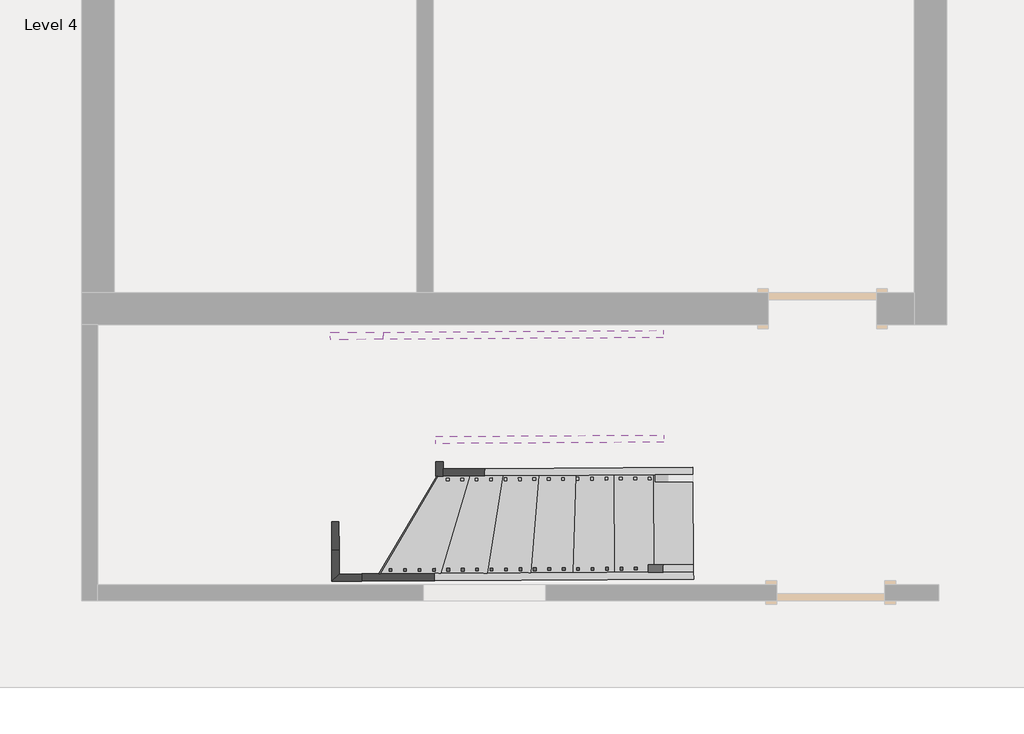
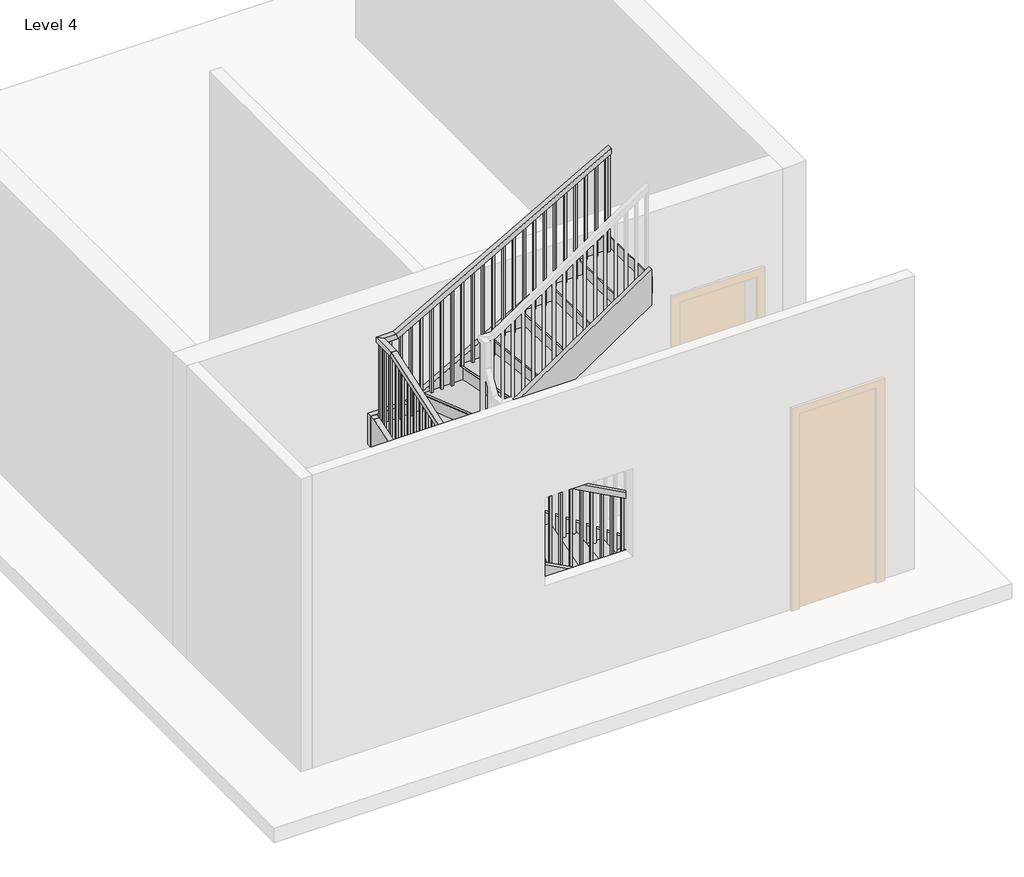
# One storey, part 2 of 2: 9 members, 1 railing, 1 stair flight.
"""IFC4 building model written with IfcOpenShell, lengths in millimetres."""

from ifc_helpers import new_model, si_unit, frame, origin, place, context, project, spatial, polyline, outline, extrude, faceted_brep, transform, mapped, element, save
from components import stair_flight_a1ba2c50

model = new_model("IFC4")

# Units and contexts
model_context = context("Model", 3, world=origin())
ifc_project = project(units=[si_unit("LENGTHUNIT", "METRE", prefix="MILLI")], contexts=[model_context])

# Site, building, storey
site = spatial("IfcSite", under=ifc_project)
building = spatial("IfcBuilding", under=site)
storey = spatial("IfcBuildingStorey", under=building, Name="Level 4", Elevation=6400.8)

# Members
placement = place(None, origin())
element("IfcMember", 1, ObjectType="Stringer - 2\" Width", at=placement, inside=storey, context=model_context, shape_type="SweptSolid", body=[
    extrude(outline(polyline([(-106.4787477, -199.0602913), (0.0, 0.0), (2650.4216713, 0.0), (2487.3820108, -304.8), (91.199922, -304.8), (-106.4787477, -199.0602913)])), frame((-116.1777511, -4276.2080688, 6626.5492487), z_axis=(-0.006129891180436155, 0.9999812120405643, 0.0), x_axis=(-0.8817595296628616, -0.0054051915166648664, 0.47166822635555733)), (0.0, 0.0, 1.0), 50.8),
])
element("IfcMember", 2, ObjectType="Stringer - 2\" Width", at=placement, inside=storey, context=model_context, shape_type="SweptSolid", body=[
    extrude(outline(polyline([(-2453.5237158, -4239.7350599), (-2453.2123174, -4290.5341055), (-2663.1420684, -4291.8209762), (-2612.6544213, -4240.7105322), (-2453.5237158, -4239.7350599)])), frame((0.0, 0.0, 7531.0029558), z_axis=(0.0, 0.0, 1.0), x_axis=(1.0, 0.0, 0.0)), (0.0, 0.0, 1.0), 345.6659817),
])
element("IfcMember", 3, ObjectType="Stringer - 2\" Width", at=placement, inside=storey, context=model_context, shape_type="SweptSolid", body=[
    extrude(outline(polyline([(-2612.6544213, -4240.7105322), (-2663.1420684, -4291.8209762), (-2664.4731567, -4074.6779247), (-2613.6741111, -4074.3665263), (-2612.6544213, -4240.7105322)])), frame((0.0, 0.0, 7531.0029558), z_axis=(0.0, 0.0, 1.0), x_axis=(1.0, 0.0, 0.0)), (0.0, 0.0, 1.0), 345.6659817),
])
element("IfcMember", 4, ObjectType="Stringer - 2\" Width", at=placement, inside=storey, context=model_context, shape_type="SweptSolid", body=[
    extrude(outline(polyline([(-112.9595567, -326.688092), (0.0, 0.0), (1516.7940002, 1e-07), (1565.1210838, -16.7101466), (1457.9394259, -326.6880919), (-112.9595567, -326.688092)])), frame((-2664.4731567, -4074.6779247, 7876.6689375), z_axis=(0.9999812120405643, 0.006129891180436421, 0.0), x_axis=(-0.005793345483301546, 0.9450798501367781, 0.3267881791215163)), (0.0, 0.0, 1.0), 50.8),
])
element("IfcMember", 5, ObjectType="Stringer - 2\" Width", at=placement, inside=storey, context=model_context, shape_type="SweptSolid", body=[
    extrude(outline(polyline([(-111.800968, -163.7049666), (0.0, 0.0), (2130.8093531, 0.0), (1922.648686, -304.8000001), (94.7979387, -304.8000001), (-111.800968, -163.7049666)])), frame((-120.6930289, -3539.621908, 6599.0391801), z_axis=(-0.006129891180436334, 0.9999812120405643, 0.0), x_axis=(-0.8257797012408892, -0.005062034812924604, 0.5639700885880922)), (0.0, 0.0, 1.0), 50.8),
])
element("IfcMember", 6, ObjectType="Stringer - 2\" Width", at=placement, inside=storey, context=model_context, shape_type="SweptSolid", body=[
    extrude(outline(polyline([(-476.3090819, -288.3824073), (0.0, 0.0), (441.380003, 0.0), (-62.0453256, -304.8), (-466.3690133, -304.8), (-476.3090819, -288.3824073)])), frame((-1931.0711854, -3550.7195376, 8023.1542381), z_axis=(0.9999812120405643, 0.006129891180436036, 0.0), x_axis=(-0.00317479975135555, 0.5179113315223286, 0.8554284150806002)), (0.0, 0.0, 1.0), 50.8),
])
element("IfcMember", 7, ObjectType="Stringer - 2\" Width", at=placement, inside=storey, context=model_context, shape_type="SweptSolid", body=[
    extrude(outline(polyline([(205.0123517, -304.8), (0.0, 0.0), (1938.1040339, 0.0), (2143.1163855, -304.8), (205.0123517, -304.8)])), frame((-1932.4724786, -3322.1238325, 8067.7006308), z_axis=(-0.006129891180436482, 0.9999812120405644, 0.0), x_axis=(0.8297505463599371, 0.005086376118722323, 0.5581112430271987)), (0.0, 0.0, 1.0), 50.8),
])
element("IfcMember", 8, ObjectType="Stringer - 2\" Width", at=placement, inside=storey, context=model_context, shape_type="SweptSolid", body=[
    extrude(outline(polyline([(-2673.5739172, -2590.0529496), (-2673.8853157, -2539.253904), (-2303.2697085, -2536.982028), (-2302.9583101, -2587.7810735), (-2673.5739172, -2590.0529496)])), frame((0.0, 0.0, 8049.8329153), z_axis=(0.0, 0.0, 1.0), x_axis=(1.0, 0.0, 0.0)), (0.0, 0.0, 1.0), 322.5063717),
])
element("IfcMember", 9, ObjectType="Stringer - 2\" Width", at=placement, inside=storey, context=model_context, shape_type="SweptSolid", body=[
    extrude(outline(polyline([(155.3220552, -282.6400873), (0.0, 0.0), (2252.6037587, 1e-07), (2407.9258139, -282.6400872), (155.3220552, -282.6400873)])), frame((-2302.9583101, -2587.7810735, 8049.8329153), z_axis=(-0.006129891180436272, 0.9999812120405644, 0.0), x_axis=(0.8763695910030255, 0.005372151158450034, 0.4816092606637882)), (0.0, 0.0, 1.0), 50.8),
])

# Railing
element("IfcRailing", 10, ObjectType="Handrail - Rectangular", at=placement, inside=storey, context=model_context, shape_type="SolidModel", body=[
    faceted_brep([(-116.4891496, -4225.4090232, 7484.5333333), (-116.4891496, -4225.4090232, 7426.7022634), (-116.800548, -4174.6099776, 7426.7022634), (-116.800548, -4174.6099776, 7484.5333333), (-2474.2717021, -4239.8622452, 8767.2653479), (-2487.1954725, -4239.941468, 8716.4653479), (-2487.506871, -4189.1424224, 8716.4653479), (-2474.5831006, -4189.0631997, 8767.2653479), (-2612.6544213, -4240.7105322, 8767.2653479), (-2612.6544213, -4240.7105322, 8716.4653479), (-2562.1667742, -4189.6000881, 8716.4653479), (-2562.1667742, -4189.6000881, 8767.2653479), (-2613.899826, -4037.5452114, 8767.2653479), (-2613.9521428, -4029.010664, 8716.4653479), (-2563.1530973, -4028.6992655, 8716.4653479), (-2563.1007804, -4037.2338129, 8767.2653479), (-2621.180916, -2849.7666717, 9177.9734867), (-2621.2332328, -2841.2321243, 9127.1734867), (-2570.4341872, -2840.9207258, 9127.1734867), (-2570.3818704, -2849.4552732, 9177.9734867), (-2622.7748716, -2589.7415511, 9177.9734867), (-2622.7748716, -2589.7415511, 9127.1734867), (-2571.6644276, -2640.2291982, 9127.1734867), (-2571.6644276, -2640.2291982, 9177.9734867), (-2452.0429693, -2588.6949634, 9177.9734867), (-2438.8245474, -2588.6139344, 9127.1734867), (-2438.513149, -2639.41298, 9127.1734867), (-2451.7315708, -2639.494009, 9177.9734867), (-328.8448754, -2575.6797456, 10363.2), (-328.533477, -2626.4787912, 10363.2), (-328.533477, -2626.4787912, 10305.02112), (-328.8448754, -2575.6797456, 10305.02112)], [[[0, 1, 2, 3]], [[1, 0, 4, 5]], [[2, 1, 5, 6]], [[3, 2, 6, 7]], [[0, 3, 7, 4]], [[5, 4, 8, 9]], [[6, 5, 9, 10]], [[7, 6, 10, 11]], [[4, 7, 11, 8]], [[9, 8, 12, 13]], [[10, 9, 13, 14]], [[11, 10, 14, 15]], [[8, 11, 15, 12]], [[13, 12, 16, 17]], [[14, 13, 17, 18]], [[15, 14, 18, 19]], [[12, 15, 19, 16]], [[17, 16, 20, 21]], [[18, 17, 21, 22]], [[19, 18, 22, 23]], [[16, 19, 23, 20]], [[21, 20, 24, 25]], [[22, 21, 25, 26]], [[23, 22, 26, 27]], [[20, 23, 27, 24]], [[28, 29, 30, 31]], [[25, 24, 28, 31]], [[26, 25, 31, 30]], [[27, 26, 30, 29]], [[24, 27, 29, 28]]]),
    extrude(outline(polyline([(233.9170124, 19.05), (1235.5250403, 19.05), (1235.5250403, 0.0), (223.2829877, 0.0), (233.9170124, 19.05)])), frame((-352.4784362, -2610.7502757, 10514.991707), z_axis=(-0.0061298911804362555, 0.9999812120405644, 0.0), x_axis=(0.0, 0.0, -1.0)), (0.0, 0.0, 1.0), 19.05),
    extrude(outline(polyline([(233.9170123, 19.05), (1178.8102421, 19.05), (1178.8102421, 0.0), (223.2829877, 0.0), (233.9170123, 19.05)])), frame((-454.0765273, -2611.3730726, 10458.2769088), z_axis=(-0.0061298911804362555, 0.9999812120405644, 0.0), x_axis=(0.0, 0.0, -1.0)), (0.0, 0.0, 1.0), 19.05),
    extrude(outline(polyline([(233.9170124, 19.05), (1122.095444, 19.05), (1122.095444, 0.0), (223.2829877, 0.0), (233.9170124, 19.05)])), frame((-555.6746185, -2611.9958696, 10401.5621107), z_axis=(-0.0061298911804362555, 0.9999812120405644, 0.0), x_axis=(0.0, 0.0, -1.0)), (0.0, 0.0, 1.0), 19.05),
    extrude(outline(polyline([(233.9170123, 19.05), (1234.7139792, 19.05), (1234.7139792, 0.0), (223.2829877, 0.0), (233.9170123, 19.05)])), frame((-657.2727096, -2612.6186665, 10344.8473125), z_axis=(-0.0061298911804362555, 0.9999812120405644, 0.0), x_axis=(0.0, 0.0, -1.0)), (0.0, 0.0, 1.0), 19.05),
    extrude(outline(polyline([(233.9170123, 19.05), (1177.999181, 19.05), (1177.999181, 0.0), (223.2829876, 0.0), (233.9170123, 19.05)])), frame((-758.8708008, -2613.2414635, 10288.1325143), z_axis=(-0.0061298911804362555, 0.9999812120405644, 0.0), x_axis=(0.0, 0.0, -1.0)), (0.0, 0.0, 1.0), 19.05),
    extrude(outline(polyline([(233.9170123, 19.05), (1121.2843829, 19.05), (1121.2843829, 0.0), (223.2829877, 0.0), (233.9170123, 19.05)])), frame((-860.4688919, -2613.8642604, 10231.4177162), z_axis=(-0.0061298911804362555, 0.9999812120405644, 0.0), x_axis=(0.0, 0.0, -1.0)), (0.0, 0.0, 1.0), 19.05),
    extrude(outline(polyline([(233.9170123, 19.0499999), (1233.902918, 19.0499999), (1233.902918, 0.0), (223.2829876, 0.0), (233.9170123, 19.0499999)])), frame((-962.0669831, -2614.4870574, 10174.702918), z_axis=(-0.0061298911804362555, 0.9999812120405644, 0.0), x_axis=(0.0, 0.0, -1.0)), (0.0, 0.0, 1.0), 19.05),
    extrude(outline(polyline([(233.9170123, 19.05), (1177.1881199, 19.05), (1177.1881199, 0.0), (223.2829877, 0.0), (233.9170123, 19.05)])), frame((-1063.6650742, -2615.1098543, 10117.9881199), z_axis=(-0.0061298911804362555, 0.9999812120405644, 0.0), x_axis=(0.0, 0.0, -1.0)), (0.0, 0.0, 1.0), 19.05),
    extrude(outline(polyline([(233.9170123, 19.05), (1120.4733217, 19.05), (1120.4733217, 0.0), (223.2829876, 0.0), (233.9170123, 19.05)])), frame((-1165.2631653, -2615.7326513, 10061.2733217), z_axis=(-0.0061298911804362555, 0.9999812120405644, 0.0), x_axis=(0.0, 0.0, -1.0)), (0.0, 0.0, 1.0), 19.05),
    extrude(outline(polyline([(233.9170123, 19.05), (1233.0918569, 19.05), (1233.0918569, 0.0), (223.2829877, 0.0), (233.9170123, 19.05)])), frame((-1266.8612565, -2616.3554482, 10004.5585236), z_axis=(-0.0061298911804362555, 0.9999812120405644, 0.0), x_axis=(0.0, 0.0, -1.0)), (0.0, 0.0, 1.0), 19.05),
    extrude(outline(polyline([(233.9170123, 19.05), (1176.3770587, 19.05), (1176.3770587, 0.0), (223.2829876, 0.0), (233.9170123, 19.05)])), frame((-1368.4593476, -2616.9782451, 9947.8437254), z_axis=(-0.0061298911804362555, 0.9999812120405644, 0.0), x_axis=(0.0, 0.0, -1.0)), (0.0, 0.0, 1.0), 19.05),
    extrude(outline(polyline([(233.9170123, 19.05), (1288.995594, 19.05), (1288.995594, 0.0), (223.2829877, 0.0), (233.9170123, 19.05)])), frame((-1470.0574388, -2617.6010421, 9891.1289273), z_axis=(-0.0061298911804362555, 0.9999812120405644, 0.0), x_axis=(0.0, 0.0, -1.0)), (0.0, 0.0, 1.0), 19.05),
    extrude(outline(polyline([(233.9170123, 19.05), (1232.2807958, 19.05), (1232.2807958, 0.0), (223.2829876, 0.0), (233.9170123, 19.05)])), frame((-1571.6555299, -2618.223839, 9834.4141291), z_axis=(-0.0061298911804362555, 0.9999812120405644, 0.0), x_axis=(0.0, 0.0, -1.0)), (0.0, 0.0, 1.0), 19.05),
    extrude(outline(polyline([(233.9170123, 19.05), (1175.5659977, 19.05), (1175.5659977, 0.0), (223.2829877, 0.0), (233.9170123, 19.05)])), frame((-1673.2536211, -2618.846636, 9777.699331), z_axis=(-0.0061298911804362555, 0.9999812120405644, 0.0), x_axis=(0.0, 0.0, -1.0)), (0.0, 0.0, 1.0), 19.05),
    extrude(outline(polyline([(233.9170123, 19.05), (1118.8511995, 19.05), (1118.8511995, 0.0), (223.2829876, 0.0), (233.9170123, 19.05)])), frame((-1774.8517122, -2619.4694329, 9720.9845328), z_axis=(-0.0061298911804362555, 0.9999812120405644, 0.0), x_axis=(0.0, 0.0, -1.0)), (0.0, 0.0, 1.0), 19.05),
    extrude(outline(polyline([(233.9170123, 19.05), (1231.4697347, 19.05), (1231.4697347, 0.0), (223.2829877, 0.0), (233.9170123, 19.05)])), frame((-1876.4498033, -2620.0922299, 9664.2697347), z_axis=(-0.0061298911804362555, 0.9999812120405644, 0.0), x_axis=(0.0, 0.0, -1.0)), (0.0, 0.0, 1.0), 19.05),
    extrude(outline(polyline([(233.9170123, 19.05), (1174.7549365, 19.05), (1174.7549365, 0.0), (223.2829876, 0.0), (233.9170123, 19.05)])), frame((-1978.0478945, -2620.7150268, 9607.5549365), z_axis=(-0.0061298911804362555, 0.9999812120405644, 0.0), x_axis=(0.0, 0.0, -1.0)), (0.0, 0.0, 1.0), 19.05),
    extrude(outline(polyline([(233.9170124, 19.05), (1118.0401384, 19.05), (1118.0401384, 0.0), (223.2829877, 0.0), (233.9170124, 19.05)])), frame((-2079.6459856, -2621.3378238, 9550.8401384), z_axis=(-0.0061298911804362555, 0.9999812120405644, 0.0), x_axis=(0.0, 0.0, -1.0)), (0.0, 0.0, 1.0), 19.05),
    extrude(outline(polyline([(233.9170123, 19.05), (1230.6586735, 19.05), (1230.6586735, 0.0), (223.2829876, 0.0), (233.9170123, 19.05)])), frame((-2181.2440768, -2621.9606207, 9494.1253402), z_axis=(-0.0061298911804362555, 0.9999812120405644, 0.0), x_axis=(0.0, 0.0, -1.0)), (0.0, 0.0, 1.0), 19.05),
    extrude(outline(polyline([(233.9170124, 19.05), (1173.9438754, 19.05), (1173.9438754, 0.0), (223.2829877, 0.0), (233.9170124, 19.05)])), frame((-2282.8421679, -2622.5834176, 9437.4105421), z_axis=(-0.0061298911804362555, 0.9999812120405644, 0.0), x_axis=(0.0, 0.0, -1.0)), (0.0, 0.0, 1.0), 19.05),
    extrude(outline(polyline([(233.9170123, 19.05), (1117.2290772, 19.05), (1117.2290772, 0.0), (223.2829877, 0.0), (233.9170123, 19.05)])), frame((-2384.4402591, -2623.2062146, 9380.6957439), z_axis=(-0.0061298911804362555, 0.9999812120405644, 0.0), x_axis=(0.0, 0.0, -1.0)), (0.0, 0.0, 1.0), 19.05),
    extrude(outline(polyline([(-2505.2047667, -2604.8961439), (-2486.1551246, -2604.7793694), (-2486.0383502, -2623.8290115), (-2505.0879923, -2623.945786), (-2505.2047667, -2604.8961439)])), frame((0.0, 0.0, 8263.4666667), z_axis=(0.0, 0.0, 1.0), x_axis=(1.0, 0.0, 0.0)), (0.0, 0.0, 1.0), 863.70682),
    extrude(outline(polyline([(-2606.2189857, -2700.7671513), (-2606.3357602, -2681.7175092), (-2587.2861181, -2681.6007347), (-2587.1693436, -2700.6503768), (-2606.2189857, -2700.7671513)])), frame((0.0, 0.0, 8263.4666667), z_axis=(0.0, 0.0, 1.0), x_axis=(1.0, 0.0, 0.0)), (0.0, 0.0, 1.0), 863.70682),
    extrude(outline(polyline([(-2605.5961888, -2802.3652424), (-2605.7129632, -2783.3156003), (-2586.6633211, -2783.1988259), (-2586.5465467, -2802.248468), (-2605.5961888, -2802.3652424)])), frame((0.0, 0.0, 8263.4666667), z_axis=(0.0, 0.0, 1.0), x_axis=(1.0, 0.0, 0.0)), (0.0, 0.0, 1.0), 863.70682),
    extrude(outline(polyline([(225.3065228, 19.0499999), (1243.2088863, 19.0499999), (1243.2088863, 0.0), (231.8934772, 0.0), (225.3065228, 19.0499999)])), frame((-2604.9733918, -2903.9633335, 9337.3422196), z_axis=(0.9999812120405643, 0.0061298911804362685, 0.0), x_axis=(0.0, 0.0, -1.0)), (0.0, 0.0, 1.0), 19.05),
    extrude(outline(polyline([(225.3065229, 19.05), (1208.078463, 19.05), (1208.078463, 0.0), (231.8934772, 0.0), (225.3065229, 19.05)])), frame((-2604.3505949, -3005.5614247, 9302.2117963), z_axis=(0.9999812120405643, 0.0061298911804362685, 0.0), x_axis=(0.0, 0.0, -1.0)), (0.0, 0.0, 1.0), 19.05),
    extrude(outline(polyline([(225.3065228, 19.05), (1172.9480396, 19.05), (1172.9480396, 0.0), (231.8934772, 0.0), (225.3065228, 19.05)])), frame((-2603.727798, -3107.1595158, 9267.0813729), z_axis=(0.9999812120405643, 0.0061298911804362685, 0.0), x_axis=(0.0, 0.0, -1.0)), (0.0, 0.0, 1.0), 19.05),
    extrude(outline(polyline([(225.3065228, 19.05), (1137.8176163, 19.05), (1137.8176163, 0.0), (231.8934772, 0.0), (225.3065228, 19.05)])), frame((-2603.105001, -3208.757607, 9231.9509496), z_axis=(0.9999812120405643, 0.0061298911804362685, 0.0), x_axis=(0.0, 0.0, -1.0)), (0.0, 0.0, 1.0), 19.05),
    extrude(outline(polyline([(225.3065228, 19.05), (1102.687193, 19.05), (1102.687193, 0.0), (231.8934772, 0.0), (225.3065228, 19.05)])), frame((-2602.4822041, -3310.3556981, 9196.8205263), z_axis=(0.9999812120405643, 0.0061298911804362685, 0.0), x_axis=(0.0, 0.0, -1.0)), (0.0, 0.0, 1.0), 19.05),
    extrude(outline(polyline([(225.3065228, 19.05), (1236.890103, 19.05), (1236.890103, 0.0), (231.8934772, 0.0), (225.3065228, 19.05)])), frame((-2601.8594071, -3411.9537893, 9161.690103), z_axis=(0.9999812120405643, 0.0061298911804362685, 0.0), x_axis=(0.0, 0.0, -1.0)), (0.0, 0.0, 1.0), 19.05),
    extrude(outline(polyline([(225.3065229, 19.05), (1201.7596797, 19.05), (1201.7596797, 0.0), (231.8934772, 0.0), (225.3065229, 19.05)])), frame((-2601.2366102, -3513.5518804, 9126.5596797), z_axis=(0.9999812120405643, 0.0061298911804362685, 0.0), x_axis=(0.0, 0.0, -1.0)), (0.0, 0.0, 1.0), 19.05),
    extrude(outline(polyline([(225.3065228, 19.0499999), (1166.6292563, 19.0499999), (1166.6292563, 0.0), (231.8934772, 0.0), (225.3065228, 19.0499999)])), frame((-2600.6138132, -3615.1499715, 9091.4292563), z_axis=(0.9999812120405643, 0.0061298911804362685, 0.0), x_axis=(0.0, 0.0, -1.0)), (0.0, 0.0, 1.0), 19.05),
    extrude(outline(polyline([(225.3065228, 19.05), (1131.498833, 19.05), (1131.498833, 0.0), (231.8934772, 0.0), (225.3065228, 19.05)])), frame((-2599.9910163, -3716.7480627, 9056.298833), z_axis=(0.9999812120405643, 0.0061298911804362685, 0.0), x_axis=(0.0, 0.0, -1.0)), (0.0, 0.0, 1.0), 19.05),
    extrude(outline(polyline([(225.3065228, 19.05), (1096.3684097, 19.05), (1096.3684097, 0.0), (231.8934772, 0.0), (225.3065228, 19.05)])), frame((-2599.3682194, -3818.3461538, 9021.1684097), z_axis=(0.9999812120405643, 0.0061298911804362685, 0.0), x_axis=(0.0, 0.0, -1.0)), (0.0, 0.0, 1.0), 19.05),
    extrude(outline(polyline([(225.3065228, 19.05), (1230.5713197, 19.05), (1230.5713197, 0.0), (231.8934772, 0.0), (225.3065228, 19.05)])), frame((-2598.7454224, -3919.944245, 8986.0379864), z_axis=(0.9999812120405643, 0.0061298911804362685, 0.0), x_axis=(0.0, 0.0, -1.0)), (0.0, 0.0, 1.0), 19.05),
    extrude(outline(polyline([(225.3065228, 19.05), (1195.4408963, 19.05), (1195.4408963, 0.0), (231.8934771, 0.0), (225.3065228, 19.05)])), frame((-2598.1226255, -4021.5423361, 8950.907563), z_axis=(0.9999812120405643, 0.0061298911804362685, 0.0), x_axis=(0.0, 0.0, -1.0)), (0.0, 0.0, 1.0), 19.05),
    extrude(outline(polyline([(-2597.4998285, -4123.1404273), (-2597.6166029, -4104.0907852), (-2578.5669609, -4103.9740107), (-2578.4501864, -4123.0236528), (-2597.4998285, -4123.1404273)])), frame((0.0, 0.0, 7755.4666667), z_axis=(0.0, 0.0, 1.0), x_axis=(1.0, 0.0, 0.0)), (0.0, 0.0, 1.0), 960.9986813),
    extrude(outline(polyline([(-2545.415828, -4224.4230609), (-2564.4654701, -4224.5398353), (-2564.5822445, -4205.4901932), (-2545.5326024, -4205.3734188), (-2545.415828, -4224.4230609)])), frame((0.0, 0.0, 7755.4666667), z_axis=(0.0, 0.0, 1.0), x_axis=(1.0, 0.0, 0.0)), (0.0, 0.0, 1.0), 960.9986813),
    extrude(outline(polyline([(223.4181002, 19.05), (1171.1283424, 19.05), (1171.1283424, 0.0), (233.7818998, 0.0), (223.4181002, 19.05)])), frame((-2443.8177368, -4223.800264, 8926.5950091), z_axis=(-0.006129891180436165, 0.9999812120405643, 0.0), x_axis=(0.0, 0.0, -1.0)), (0.0, 0.0, 1.0), 19.05),
    extrude(outline(polyline([(223.4181002, 19.05), (1115.8547448, 19.05), (1115.8547448, 0.0), (233.7818998, 0.0), (223.4181002, 19.05)])), frame((-2342.2196457, -4223.177467, 8871.3214115), z_axis=(-0.006129891180436165, 0.9999812120405643, 0.0), x_axis=(0.0, 0.0, -1.0)), (0.0, 0.0, 1.0), 19.05),
    extrude(outline(polyline([(223.4181002, 19.05), (1229.9144805, 19.05), (1229.9144805, 0.0), (233.7818997, 0.0), (223.4181002, 19.05)])), frame((-2240.6215545, -4222.5546701, 8816.0478138), z_axis=(-0.006129891180436165, 0.9999812120405643, 0.0), x_axis=(0.0, 0.0, -1.0)), (0.0, 0.0, 1.0), 19.05),
    extrude(outline(polyline([(223.4181002, 19.05), (1174.6408829, 19.05), (1174.6408829, 0.0), (233.7818998, 0.0), (223.4181002, 19.05)])), frame((-2139.0234634, -4221.9318731, 8760.7742162), z_axis=(-0.006129891180436165, 0.9999812120405643, 0.0), x_axis=(0.0, 0.0, -1.0)), (0.0, 0.0, 1.0), 19.05),
    extrude(outline(polyline([(223.4181003, 19.0499999), (1119.3672853, 19.0499999), (1119.3672853, 0.0), (233.7818998, 0.0), (223.4181003, 19.0499999)])), frame((-2037.4253723, -4221.3090762, 8705.5006186), z_axis=(-0.006129891180436165, 0.9999812120405643, 0.0), x_axis=(0.0, 0.0, -1.0)), (0.0, 0.0, 1.0), 19.05),
    extrude(outline(polyline([(223.4181002, 19.05), (1064.0936876, 19.05), (1064.0936876, 0.0), (233.7818998, 0.0), (223.4181002, 19.05)])), frame((-1935.8272811, -4220.6862792, 8650.2270209), z_axis=(-0.006129891180436165, 0.9999812120405643, 0.0), x_axis=(0.0, 0.0, -1.0)), (0.0, 0.0, 1.0), 19.05),
    extrude(outline(polyline([(223.4181002, 19.05), (1178.1534233, 19.05), (1178.1534233, 0.0), (233.7818998, 0.0), (223.4181002, 19.05)])), frame((-1834.22919, -4220.0634823, 8594.9534233), z_axis=(-0.006129891180436165, 0.9999812120405643, 0.0), x_axis=(0.0, 0.0, -1.0)), (0.0, 0.0, 1.0), 19.05),
    extrude(outline(polyline([(223.4181002, 19.05), (1122.8798256, 19.05), (1122.8798256, 0.0), (233.7818997, 0.0), (223.4181002, 19.05)])), frame((-1732.6310988, -4219.4406854, 8539.6798256), z_axis=(-0.006129891180436165, 0.9999812120405643, 0.0), x_axis=(0.0, 0.0, -1.0)), (0.0, 0.0, 1.0), 19.05),
    extrude(outline(polyline([(223.4181002, 19.05), (1067.606228, 19.05), (1067.606228, 0.0), (233.7818998, 0.0), (223.4181002, 19.05)])), frame((-1631.0330077, -4218.8178884, 8484.406228), z_axis=(-0.006129891180436165, 0.9999812120405643, 0.0), x_axis=(0.0, 0.0, -1.0)), (0.0, 0.0, 1.0), 19.05),
    extrude(outline(polyline([(223.4181003, 19.05), (1181.6659637, 19.05), (1181.6659637, 0.0), (233.7818998, 0.0), (223.4181003, 19.05)])), frame((-1529.4349165, -4218.1950915, 8429.1326304), z_axis=(-0.006129891180436165, 0.9999812120405643, 0.0), x_axis=(0.0, 0.0, -1.0)), (0.0, 0.0, 1.0), 19.05),
    extrude(outline(polyline([(223.4181002, 19.05), (1126.392366, 19.05), (1126.392366, 0.0), (233.7818998, 0.0), (223.4181002, 19.05)])), frame((-1427.8368254, -4217.5722945, 8373.8590327), z_axis=(-0.006129891180436165, 0.9999812120405643, 0.0), x_axis=(0.0, 0.0, -1.0)), (0.0, 0.0, 1.0), 19.05),
    extrude(outline(polyline([(223.4181002, 19.0499999), (1071.1187684, 19.0499999), (1071.1187684, 0.0), (233.7818998, 0.0), (223.4181002, 19.0499999)])), frame((-1326.2387343, -4216.9494976, 8318.5854351), z_axis=(-0.006129891180436165, 0.9999812120405643, 0.0), x_axis=(0.0, 0.0, -1.0)), (0.0, 0.0, 1.0), 19.05),
    extrude(outline(polyline([(223.4181002, 19.05), (1185.1785041, 19.05), (1185.1785041, 0.0), (233.7818997, 0.0), (223.4181002, 19.05)])), frame((-1224.6406431, -4216.3267006, 8263.3118374), z_axis=(-0.006129891180436165, 0.9999812120405643, 0.0), x_axis=(0.0, 0.0, -1.0)), (0.0, 0.0, 1.0), 19.05),
    extrude(outline(polyline([(223.4181002, 19.05), (1129.9049065, 19.05), (1129.9049065, 0.0), (233.7818998, 0.0), (223.4181002, 19.05)])), frame((-1123.042552, -4215.7039037, 8208.0382398), z_axis=(-0.006129891180436165, 0.9999812120405643, 0.0), x_axis=(0.0, 0.0, -1.0)), (0.0, 0.0, 1.0), 19.05),
    extrude(outline(polyline([(223.4181003, 19.05), (1074.6313089, 19.05), (1074.6313089, 0.0), (233.7818998, 0.0), (223.4181003, 19.05)])), frame((-1021.4444608, -4215.0811067, 8152.7646422), z_axis=(-0.006129891180436165, 0.9999812120405643, 0.0), x_axis=(0.0, 0.0, -1.0)), (0.0, 0.0, 1.0), 19.05),
    extrude(outline(polyline([(223.4181002, 19.05), (1188.6910445, 19.05), (1188.6910445, 0.0), (233.7818998, 0.0), (223.4181002, 19.05)])), frame((-919.8463697, -4214.4583098, 8097.4910445), z_axis=(-0.006129891180436165, 0.9999812120405643, 0.0), x_axis=(0.0, 0.0, -1.0)), (0.0, 0.0, 1.0), 19.05),
    extrude(outline(polyline([(223.4181002, 19.05), (1133.4174469, 19.05), (1133.4174469, 0.0), (233.7818998, 0.0), (223.4181002, 19.05)])), frame((-818.2482785, -4213.8355129, 8042.2174469), z_axis=(-0.006129891180436165, 0.9999812120405643, 0.0), x_axis=(0.0, 0.0, -1.0)), (0.0, 0.0, 1.0), 19.05),
    extrude(outline(polyline([(223.4181002, 19.05), (1078.1438492, 19.05), (1078.1438492, 0.0), (233.7818997, 0.0), (223.4181002, 19.05)])), frame((-716.6501874, -4213.2127159, 7986.9438492), z_axis=(-0.006129891180436165, 0.9999812120405643, 0.0), x_axis=(0.0, 0.0, -1.0)), (0.0, 0.0, 1.0), 19.05),
    extrude(outline(polyline([(223.4181002, 19.0499999), (1192.2035849, 19.0499999), (1192.2035849, 0.0), (233.7818998, 0.0), (223.4181002, 19.0499999)])), frame((-615.0520963, -4212.589919, 7931.6702516), z_axis=(-0.006129891180436165, 0.9999812120405643, 0.0), x_axis=(0.0, 0.0, -1.0)), (0.0, 0.0, 1.0), 19.05),
    extrude(outline(polyline([(223.4181003, 19.05), (1136.9299873, 19.05), (1136.9299873, 0.0), (233.7818998, 0.0), (223.4181003, 19.05)])), frame((-513.4540051, -4211.967122, 7876.396654), z_axis=(-0.006129891180436165, 0.9999812120405643, 0.0), x_axis=(0.0, 0.0, -1.0)), (0.0, 0.0, 1.0), 19.05),
    extrude(outline(polyline([(223.4181002, 19.05), (1081.6563896, 19.05), (1081.6563896, 0.0), (233.7818998, 0.0), (223.4181002, 19.05)])), frame((-411.855914, -4211.3443251, 7821.1230563), z_axis=(-0.006129891180436165, 0.9999812120405643, 0.0), x_axis=(0.0, 0.0, -1.0)), (0.0, 0.0, 1.0), 19.05),
    extrude(outline(polyline([(223.4181002, 19.05), (1195.7161254, 19.05), (1195.7161254, 0.0), (233.7818998, 0.0), (223.4181002, 19.05)])), frame((-310.2578228, -4210.7215281, 7765.8494587), z_axis=(-0.006129891180436165, 0.9999812120405643, 0.0), x_axis=(0.0, 0.0, -1.0)), (0.0, 0.0, 1.0), 19.05),
    extrude(outline(polyline([(223.4181002, 19.05), (1140.4425277, 19.05), (1140.4425277, 0.0), (233.7818997, 0.0), (223.4181002, 19.05)])), frame((-208.6597317, -4210.0987312, 7710.575861), z_axis=(-0.006129891180436165, 0.9999812120405643, 0.0), x_axis=(0.0, 0.0, -1.0)), (0.0, 0.0, 1.0), 19.05),
    extrude(outline(polyline([(-2606.6860834, -2624.5685829), (-2606.8028579, -2605.5189408), (-2587.7532158, -2605.4021664), (-2587.6364414, -2624.4518085), (-2606.6860834, -2624.5685829)])), frame((0.0, 0.0, 8263.4666667), z_axis=(0.0, 0.0, 1.0), x_axis=(1.0, 0.0, 0.0)), (0.0, 0.0, 1.0), 863.70682),
    extrude(outline(polyline([(-2577.8273895, -4224.621744), (-2596.8770316, -4224.7385184), (-2596.993806, -4205.6888763), (-2577.9441639, -4205.5721019), (-2577.8273895, -4224.621744)])), frame((0.0, 0.0, 7755.4666667), z_axis=(0.0, 0.0, 1.0), x_axis=(1.0, 0.0, 0.0)), (0.0, 0.0, 1.0), 960.9986813),
    extrude(outline(polyline([(233.9170123, 19.05), (1248.8374409, 19.05), (1248.8374409, 0.0), (223.2829876, 0.0), (233.9170123, 19.05)])), frame((-328.630789, -2610.6040895, 10528.3041076), z_axis=(-0.0061298911804362555, 0.9999812120405644, 0.0), x_axis=(0.0, 0.0, -1.0)), (0.0, 0.0, 1.0), 19.05),
    extrude(outline(polyline([(223.4181002, 19.05), (1090.3508299, 19.05), (1090.3508299, 0.0), (233.7818998, 0.0), (223.4181002, 19.05)])), frame((-116.5864616, -4209.5343215, 7660.4841632), z_axis=(-0.006129891180436165, 0.9999812120405643, 0.0), x_axis=(0.0, 0.0, -1.0)), (0.0, 0.0, 1.0), 19.05),
])

# Stair flight
stair_flight_shape = stair_flight_a1ba2c50(model_context)
element("IfcStairFlight", 11, ObjectType="2\" Tread 1\" Nosing 1/4\" Riser", at=placement, inside=storey, context=model_context, shape_type="MappedRepresentation", body=[
    mapped(stair_flight_shape, transform((0.0, 0.0, 0.0), x_axis=(1.0, 0.0, 0.0), y_axis=(0.0, 1.0, 0.0), z_axis=(0.0, 0.0, 1.0))),
])

save(model, "model.ifc")

# Revit data of these elements
# Type "Handrail - Rectangular"
#   Assembly Code = "C2010400"
#   built-in parameter 1008612 = 0.0416667 (stored number, unit not read)
#   built-in parameter 1008611 = 0.0416667 (stored number, unit not read)
#   built-in parameter 1008609 = 0.333333 (stored number, unit not read)
#   built-in parameter 1008604 = 0.166667 (stored number, unit not read)
#   built-in parameter 1008603 = 0.166667 (stored number, unit not read)
#   Railing Height = 3' - 0"
#   built-in parameter 1008630 = 2
#   built-in parameter 1008610 = 2
#   built-in parameter 1008618 = Baluster - Square : 3/4"
# Elements 1, 2, 3, 4, 5, 6, 7, 8, 9 (IfcMember, "Stringer - 2\" Width")
#   Phase Created = New Construction
# Element 10 (IfcRailing, "Handrail - Rectangular")
#   Phase Created = New Construction
# Element 11 (IfcStairFlight, "2\" Tread 1\" Nosing 1/4\" Riser")
#   Phase Created = New Construction
